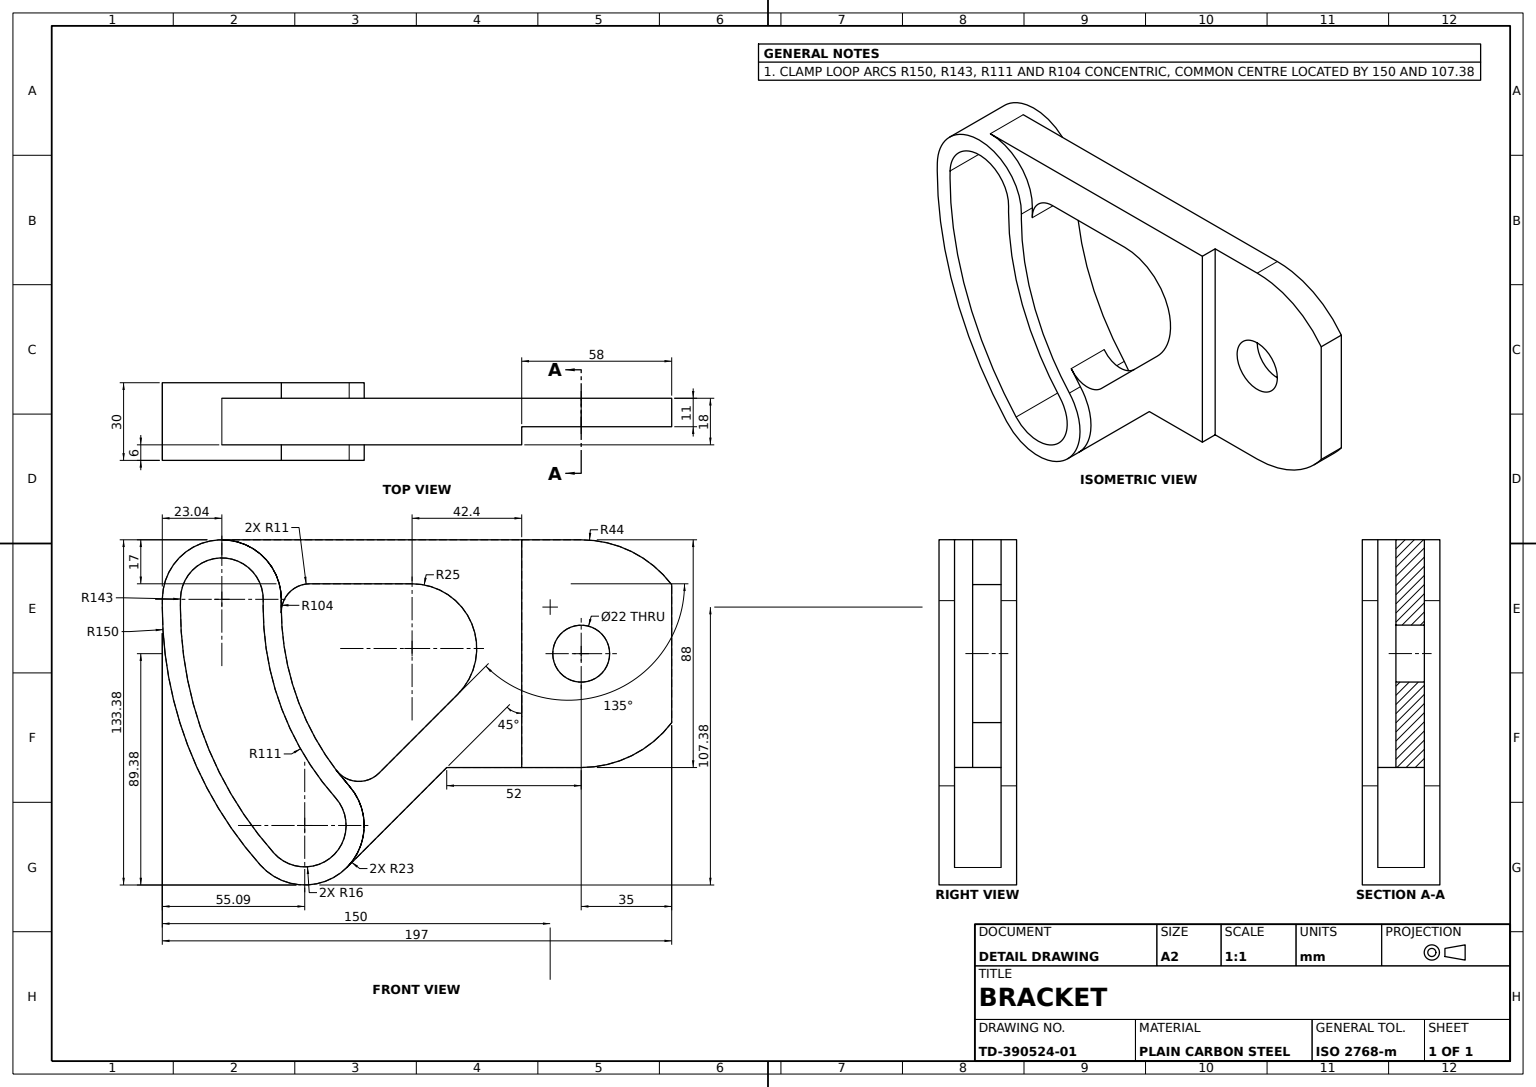
from build123d import *

# Parameters (mm, degrees)
CLAMP_LOOP_30MM_DEPTH   = 15
SUPPORT_WEB_18MM_DEPTH  = 9
MOUNTING_LUG_DEPTH      = 2
MOUNTING_LUG_DEPTH_BACK = 9
SKETCH1_4_R             = 11


with BuildPart() as part:
    # Bracket Profile Sketch → Clamp Loop 30mm (new, symmetric)
    with BuildSketch(Plane.XY):
        with BuildLine():
            ThreePointArc((-161.958144077, 21.543307087), (-152.82526794, -33.65504728), (-124.10035648, -81.666995927))
            ThreePointArc((-124.10035648, -81.666995927), (-91.629362444, -83.573444545), (-89.722913826, -51.102450509))
            ThreePointArc((-89.722913826, -51.102450509), (-109.638852439, -17.814166114), (-115.970979893, 20.456692913))
            ThreePointArc((-115.970979893, 20.456692913), (-138.421254898, 43.993582092), (-161.958144077, 21.543307087))
        make_face()
        with BuildLine():
            ThreePointArc((-122.969026617, 20.622047244), (-138.586609229, 36.995535368), (-154.960097353, 21.377952756))
            ThreePointArc((-154.960097353, 21.377952756), (-146.253422103, -31.244478407), (-118.869006511, -77.01586945))
            ThreePointArc((-118.869006511, -77.01586945), (-96.280488921, -78.342094576), (-94.954263795, -55.753576986))
            ThreePointArc((-94.954263795, -55.753576986), (-116.210698276, -20.224734987), (-122.969026617, 20.622047244))
        make_face(mode=Mode.SUBTRACT)
    extrude(amount=CLAMP_LOOP_30MM_DEPTH, both=True)

    # Sketch1_3 → Support Web 18mm (add, symmetric)
    with BuildSketch(Plane.XY):
        with BuildLine():
            Line((-23, -44), (-23, 44))
            Line((-23, 44), (-138.964561985, 44))
            ThreePointArc((-138.964561985, 44), (-122.51013913, 37.070219927), (-115.970979893, 20.456692913))
            ThreePointArc((-115.970979893, 20.456692913), (-115.999941726, 18.110094916), (-115.975948196, 15.76344086))
            ThreePointArc((-115.975948196, 15.76344086), (-112.839858129, 23.694083749), (-104.978492137, 27))
            Line((-104.978492137, 27), (-65.39696962, 27))
            ThreePointArc((-65.39696962, 27), (-42.299981307, 11.567085809), (-47.71930009, -15.67766953))
            Line((-47.71930009, -15.67766953), (-78.190423053, -46.148792492))
            ThreePointArc((-78.190423053, -46.148792492), (-86.706172416, -49.345862018), (-94.717571561, -45.038110339))
            ThreePointArc((-94.717571561, -45.038110339), (-92.277527324, -48.11746068), (-89.722913826, -51.102450509))
            ThreePointArc((-89.722913826, -51.102450509), (-83.921522259, -67.059044464), (-90.648179186, -82.648179186))
            Line((-90.648179186, -82.648179186), (-52, -44))
            Line((-52, -44), (-23, -44))
        make_face()
    extrude(amount=SUPPORT_WEB_18MM_DEPTH, both=True)

    # Sketch1_4 → Mounting Lug (add, two sides: drawn at the far end of the back side and taken through both)
    with BuildSketch(Plane.XY.offset(-MOUNTING_LUG_DEPTH_BACK)):
        with BuildLine():
            ThreePointArc((35, 26.664583252), (19.528931575, 39.428680317), (0, 44))
            Line((0, 44), (-23, 44))
            Line((-23, 44), (-23, -44))
            Line((-23, -44), (0, -44))
            ThreePointArc((0, -44), (19.528931575, -39.428680317), (35, -26.664583252))
            Line((35, -26.664583252), (35, 26.664583252))
        make_face()
        Circle(SKETCH1_4_R, mode=Mode.SUBTRACT)
    extrude(amount=MOUNTING_LUG_DEPTH + MOUNTING_LUG_DEPTH_BACK)


solid = part.part
